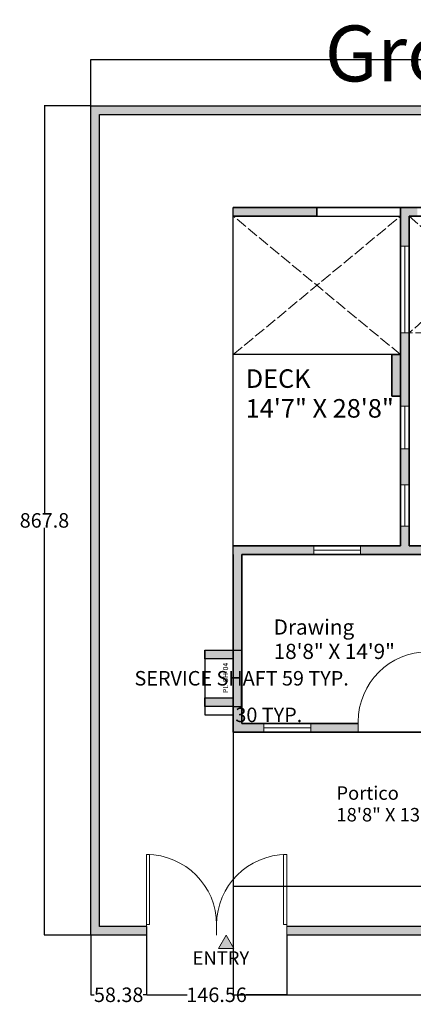
# Model space of a CAD drawing. Units: inches. Extents: x -828 to 1568, y -491 to 539.
# Tile 1 of 6: x -828 to -416, y -491 to 539. Entities that reach past the tile are written whole.
import ezdxf

# ---------------------------------------------------------------- set-up
doc = ezdxf.new("R2010")
doc.units = ezdxf.units.IN
doc.header["$MEASUREMENT"] = 0
doc.linetypes.add('ACAD_ISO02W100', pattern=[15, 12, -3])
for name, color, linetype, lineweight in [('A-ANNO-DIMS', 2, 'Continuous', 18), ('A-ANNO-SYMB', 7, 'Continuous', 18), ('A-ANNO-TEXT', 7, 'Continuous', 18), ('A-ANNO-TITL', 7, 'Continuous', 35), ('A-AREA-IDEN', 7, 'Continuous', 18), ('A-DOOR', 3, 'Continuous', 18), ('A-FLOR-EDGE', 7, 'Continuous', 25), ('A-FLOR-OVHD', 116, 'ACAD_ISO02W100', 13), ('A-FLOR-SHFT', 7, 'Continuous', 25), ('A-GLAZ', 4, 'Continuous', 18), ('A-WALL', 7, 'Continuous', 35), ('A-WALL-PATT', 8, 'Continuous', 13), ('L-SITE-GATE', 3, 'Continuous', 18), ('L-SITE-PATT', 8, 'Continuous', 13), ('L-SITE-WALL', 7, 'Continuous', 30)]:
    doc.layers.add(name, color=color, linetype=linetype, lineweight=lineweight)
doc.styles.get("Standard").update_dxf_attribs({"font": 'arial.ttf'})
doc.dimstyles.get("Standard").update_dxf_attribs({"dimtxt": 15.18, "dimasz": 0.18, "dimexe": 0.18, "dimexo": 0.0625, "dimgap": 0.09, "dimtad": 0, "dimtih": 1, "dimtoh": 1, "dimdec": 0, "dimzin": 0, "dimdsep": 46, "dimlunit": 3, "dimtxsty": 'Standard', "dimcen": 0.09, "dimadec": 0, "dimazin": 0, "dimtfac": 1, "dimtdec": 0, "dimtofl": 0, "dimtmove": 0, "dimatfit": 3, "dimfxl": 1, "dimtolj": 1, "dimtzin": 0, "dimarcsym": 0})

# ---------------------------------------------------------------- blocks, each defined once
blk = doc.blocks.new('*U2')
for p, q in [((0, 0), (0, -6)), ((40, 0), (40, -6))]:
    blk.add_line(p, q)
blk.add_lwpolyline([(0, 0), (0, 40), (1.75, 40), (1.75, 0)], close=True)
blk.add_arc((0, 0), 40, 0, 90)
blk = doc.blocks.new('SERVICE-SHAFT-59')
for p, q in [((0, 49.8), (0, 59)), ((0, 59), (29.6, 59)), ((0, 59), (0, 0)), ((29.6, 49.8), (0, 49.8)), ((0, 0), (0, 9)), ((0, 9), (29.6, 9)), ((29.6, 0), (0, 0))]:
    blk.add_line(p, q)
blk = doc.blocks.new('*D21')
at = {"layer": 'A-ANNO-DIMS', "color": 0, "lineweight": -2, "transparency": 16777216}
for p, q in [((-604.5, -120.5), (-595.5, -120.5)), ((-595.7, -120.6), (-595.7, -142)), ((-595.7, -179.3), (-595.7, -157.9)), ((-604.5, -179.4), (-595.5, -179.4))]:
    blk.add_line(p, q, dxfattribs=at)
at = {"layer": 'A-ANNO-DIMS', "color": 0, "lineweight": 20, "transparency": 16777216}
for points in [[(-595.7, -120.6), (-595.7, -120.6), (-595.7, -120.5)], [(-595.7, -179.3), (-595.7, -179.3), (-595.7, -179.4)]]:
    blk.add_solid(points, dxfattribs=at)
at = {"layer": 'DEFPOINTS', "color": 0, "lineweight": 20, "transparency": 16777216}
for p in [(-604.5, -120.5), (-595.7, -120.5), (-604.5, -179.4)]:
    blk.add_point(p, dxfattribs=at)
at = {"layer": 'A-ANNO-DIMS', "color": 0, "transparency": 16777216, "insert": (-595.7, -150), "char_height": 15.18, "attachment_point": 5}
blk.add_mtext('\\A1;SERVICE SHAFT 59 TYP.', dxfattribs=at)
blk = doc.blocks.new('*D22')
at = {"layer": 'A-ANNO-DIMS', "color": 0, "lineweight": -2, "transparency": 16777216}
for p, q in [((-634.1, -179.5), (-634.1, -188.5)), ((-604.5, -179.5), (-604.5, -188.5)), ((-633.9, -188.3), (-604.7, -188.3)), ((-604.5, -188.3), (-604.4, -188.3))]:
    blk.add_line(p, q, dxfattribs=at)
at = {"layer": 'A-ANNO-DIMS', "color": 0, "lineweight": 20, "transparency": 16777216}
for points in [[(-633.9, -188.3), (-633.9, -188.3), (-634.1, -188.3)], [(-604.7, -188.3), (-604.7, -188.3), (-604.5, -188.3)]]:
    blk.add_solid(points, dxfattribs=at)
at = {"layer": 'DEFPOINTS', "color": 0, "lineweight": 20, "transparency": 16777216}
for p in [(-634.1, -179.4), (-604.5, -179.4), (-604.5, -188.3)]:
    blk.add_point(p, dxfattribs=at)
at = {"layer": 'A-ANNO-DIMS', "color": 0, "transparency": 16777216, "insert": (-567.3, -188.3), "char_height": 15.18, "attachment_point": 5}
blk.add_mtext('\\A1;30 TYP.', dxfattribs=at)
blk = doc.blocks.new('*D31')
at = {"layer": 'A-ANNO-DIMS', "color": 0, "lineweight": -2, "transparency": 16777216}
for p, q in [((-753.5, 449.1), (-753.5, 497.6)), ((-753.3, 497.4), (-321.9, 497.4)), ((143.3, 497.4), (-288.2, 497.4)), ((143.5, 449.1), (143.5, 497.6))]:
    blk.add_line(p, q, dxfattribs=at)
at = {"layer": 'A-ANNO-DIMS', "color": 0, "lineweight": 20, "transparency": 16777216}
for points in [[(-753.3, 497.5), (-753.3, 497.4), (-753.5, 497.4)], [(143.3, 497.5), (143.3, 497.4), (143.5, 497.4)]]:
    blk.add_solid(points, dxfattribs=at)
at = {"layer": 'DEFPOINTS', "color": 0, "lineweight": 20, "transparency": 16777216}
for p in [(143.5, 497.4), (-753.5, 449), (143.5, 449)]:
    blk.add_point(p, dxfattribs=at)
at = {"layer": 'A-ANNO-DIMS', "color": 0, "transparency": 16777216, "insert": (-305, 497.4), "char_height": 15.18, "attachment_point": 5}
blk.add_mtext('\\A1;897', dxfattribs=at)
blk = doc.blocks.new('*D32')
at = {"layer": 'A-ANNO-DIMS', "color": 0, "lineweight": -2, "transparency": 16777216}
for p, q in [((-753.6, 449), (-802.1, 449)), ((-801.9, 448.9), (-801.9, 23)), ((-801.9, -418.6), (-801.9, 7.3)), ((-753.6, -418.7), (-802.1, -418.7))]:
    blk.add_line(p, q, dxfattribs=at)
at = {"layer": 'A-ANNO-DIMS', "color": 0, "lineweight": 20, "transparency": 16777216}
for points in [[(-801.9, 448.9), (-801.9, 448.9), (-801.9, 449)], [(-801.9, -418.6), (-801.9, -418.6), (-801.9, -418.7)]]:
    blk.add_solid(points, dxfattribs=at)
at = {"layer": 'DEFPOINTS', "color": 0, "lineweight": 20, "transparency": 16777216}
for p in [(-801.9, 449), (-753.5, 449), (-753.5, -418.7)]:
    blk.add_point(p, dxfattribs=at)
at = {"layer": 'A-ANNO-DIMS', "color": 0, "transparency": 16777216, "insert": (-801.9, 15.2), "char_height": 15.18, "attachment_point": 5}
blk.add_mtext('\\A1;867.8', dxfattribs=at)
blk = doc.blocks.new('*D33')
at = {"layer": 'A-ANNO-DIMS', "color": 0, "lineweight": -2, "transparency": 16777216}
for p, q in [((-604.5, -367.5), (-604.5, -481.4)), ((26.5, -367.5), (26.5, -481.4)), ((-604.4, -481.2), (-304.5, -481.2)), ((26.3, -481.2), (-273.6, -481.2))]:
    blk.add_line(p, q, dxfattribs=at)
at = {"layer": 'A-ANNO-DIMS', "color": 0, "lineweight": 20, "transparency": 16777216}
for points in [[(-604.4, -481.2), (-604.4, -481.2), (-604.5, -481.2)], [(26.3, -481.2), (26.3, -481.2), (26.5, -481.2)]]:
    blk.add_solid(points, dxfattribs=at)
at = {"layer": 'DEFPOINTS', "color": 0, "lineweight": 20, "transparency": 16777216}
for p in [(-604.5, -367.4), (26.5, -367.4), (26.5, -481.2)]:
    blk.add_point(p, dxfattribs=at)
at = {"layer": 'A-ANNO-DIMS', "color": 0, "transparency": 16777216, "insert": (-289, -481.2), "char_height": 15.18, "attachment_point": 5}
blk.add_mtext('\\A1;631', dxfattribs=at)
blk = doc.blocks.new('*D37')
at = {"layer": 'A-ANNO-DIMS', "color": 0, "lineweight": -2, "transparency": 16777216}
for p, q in [((-695.1, -418.8), (-695.1, -481.4)), ((-548.6, -418.8), (-548.6, -481.4)), ((-695, -481.2), (-652.7, -481.2)), ((-548.8, -481.2), (-591, -481.2))]:
    blk.add_line(p, q, dxfattribs=at)
at = {"layer": 'A-ANNO-DIMS', "color": 0, "lineweight": 20, "transparency": 16777216}
for points in [[(-695, -481.2), (-695, -481.2), (-695.1, -481.2)], [(-548.8, -481.2), (-548.8, -481.2), (-548.6, -481.2)]]:
    blk.add_solid(points, dxfattribs=at)
at = {"layer": 'DEFPOINTS', "color": 0, "lineweight": 20, "transparency": 16777216}
for p in [(-695.1, -418.7), (-548.6, -418.7), (-548.6, -481.2)]:
    blk.add_point(p, dxfattribs=at)
at = {"layer": 'A-ANNO-DIMS', "color": 0, "transparency": 16777216, "insert": (-621.9, -481.2), "char_height": 15.18, "attachment_point": 5}
blk.add_mtext('\\A1;146.56', dxfattribs=at)
blk = doc.blocks.new('*D38')
at = {"layer": 'A-ANNO-DIMS', "color": 0, "lineweight": -2, "transparency": 16777216}
for p, q in [((-753.5, -418.8), (-753.5, -481.4)), ((-695.1, -418.8), (-695.1, -481.4)), ((-753.3, -481.2), (-750, -481.2)), ((-695.3, -481.2), (-698.6, -481.2))]:
    blk.add_line(p, q, dxfattribs=at)
at = {"layer": 'A-ANNO-DIMS', "color": 0, "lineweight": 20, "transparency": 16777216}
for points in [[(-753.3, -481.2), (-753.3, -481.2), (-753.5, -481.2)], [(-695.3, -481.2), (-695.3, -481.2), (-695.1, -481.2)]]:
    blk.add_solid(points, dxfattribs=at)
at = {"layer": 'DEFPOINTS', "color": 0, "lineweight": 20, "transparency": 16777216}
for p in [(-753.5, -418.7), (-695.1, -418.7), (-695.1, -481.2)]:
    blk.add_point(p, dxfattribs=at)
at = {"layer": 'A-ANNO-DIMS', "color": 0, "transparency": 16777216, "insert": (-724.3, -481.2), "char_height": 15.18, "attachment_point": 5}
blk.add_mtext('\\A1;58.38', dxfattribs=at)

msp = doc.modelspace()

# ---------------------------------------------------------------- hatches: boundary and pattern name
at = {"layer": 'A-ANNO-SYMB'}
h = msp.add_hatch(color=256, dxfattribs=at)
h.dxf.hatch_style = 1
h.paths.add_polyline_path([(-611.9024, -418.9253), (-619.9125, -432.7993), (-603.8922, -432.7993)])
at = {"layer": 'A-WALL-PATT'}
h = msp.add_hatch(color=256, dxfattribs=at)
h.dxf.hatch_style = 1
h.paths.add_polyline_path([(-473.7903, -197.4155), (-523.4337, -197.4155), (-523.4337, -206.4155), (-473.7903, -206.4155)])
h.paths.add_polyline_path([(-572.3651, -197.4155), (-595.5391, -197.4155), (-595.5391, -20.4155), (-520.2134, -20.4155), (-520.2134, -11.4155), (-604.5391, -11.4155), (-604.5391, -206.4155), (-572.3651, -206.4155)])
h.paths.add_polyline_path([(-604.5391, -170.4394), (-634.1027, -170.4394), (-634.1027, -179.4394), (-604.5391, -179.4394)])
h.paths.add_polyline_path([(-604.5391, -120.4631), (-634.1027, -120.4631), (-634.1027, -129.6673), (-604.5391, -129.6673)])
h.paths.add_polyline_path([(-268.3198, -11.4155), (-420.5391, -11.4155), (-420.5391, 9.0334), (-429.5391, 9.0334), (-429.5391, -11.4155), (-471.2821, -11.4155), (-471.2821, -20.4155), (-371.5391, -20.4155), (-371.5391, -197.4155), (-400.5108, -197.4155), (-400.5108, -206.4155), (-371.5391, -206.4155), (-371.5391, -282.4155), (-367.0391, -282.4155), (-362.5391, -282.4155), (-362.5391, -122.4155), (-313.1564, -122.4155), (-313.1564, -113.4155), (-362.5391, -113.4155), (-362.5391, -20.4155), (-268.3198, -20.4155)])
h.paths.add_polyline_path([(-313.539, 165.5845), (-375.5295, 165.5845), (-375.5295, 159.5845), (-313.539, 159.5845)])
h.paths.add_polyline_path([(-420.5391, 90.211), (-429.5391, 90.211), (-429.5391, 52.4437), (-420.5391, 52.4437)])
h.paths.add_polyline_path([(-420.5391, 211.3197), (-429.5391, 211.3197), (-429.5391, 134.8496), (-425.0391, 134.8496), (-420.5391, 134.8496), (-420.5391, 165.5845)])
h.paths.add_polyline_path([(-429.5391, 188.7113), (-438.5391, 188.7113), (-438.5391, 145.3797), (-429.5391, 145.3797)])
h.paths.add_polyline_path([(-517.0391, 342.5845), (-604.5391, 342.5845), (-604.5391, 333.5845), (-517.0391, 333.5845)])
h.paths.add_polyline_path([(-411.8784, 342.5845), (-429.5391, 342.5845), (-429.5391, 302.1645), (-420.5391, 302.1645), (-420.5391, 333.5845), (-411.8784, 333.5845)])
h.paths.add_polyline_path([(-311.8294, 372.1481), (-321.0336, 372.1481), (-321.0336, 342.5845), (-311.8294, 342.5845)])
h.paths.add_polyline_path([(-282.0163, 372.1481), (-291.2206, 372.1481), (-291.2206, 342.5845), (-282.0163, 342.5845)])
h.paths.add_polyline_path([(-230.7265, 342.5845), (-321.0336, 342.5845), (-321.0336, 333.5845), (-230.7265, 333.5845)])
h.paths.add_polyline_path([(-23.3113, 372.1481), (-32.5155, 372.1481), (-32.5155, 342.5845), (-23.3113, 342.5845)])
h.paths.add_polyline_path([(26.4609, 372.1481), (17.4609, 372.1481), (17.4609, 342.5845), (26.4609, 342.5845)])
h.paths.add_polyline_path([(56.6461, 259.1031), (26.4609, 259.1031), (26.4609, 248.5663), (56.6461, 248.5663)])
h.paths.add_polyline_path([(56.6461, 216.517), (26.4609, 216.517), (26.4609, 206.4193), (56.6461, 206.4193)])
h.paths.add_polyline_path([(56.0244, -54.4391), (26.4609, -54.4391), (26.4609, -63.6433), (56.0244, -63.6433)])
h.paths.add_polyline_path([(56.0244, -163.1876), (26.4609, -163.1876), (26.4609, -172.3918), (56.0244, -172.3918)])
h.paths.add_polyline_path([(56.0244, -113.4155), (56.0244, -104.4155), (26.4609, -104.4155), (26.4609, -122.4155), (56.0244, -122.4155)])
h.paths.add_polyline_path([(-23.844, -367.4155), (-134.8372, -367.4155), (-134.8372, -376.4155), (-23.844, -376.4155)])
h.paths.add_polyline_path([(26.4609, -54.4391), (21.9609, -54.4391), (17.4609, -54.4391), (17.4609, -113.4155), (-252.861, -113.4155), (-252.861, -122.4155), (-69.5391, -122.4155), (-69.5391, -282.9566), (-65.5391, -282.9566), (-65.5391, -250.4155), (-53.4738, -250.4155), (-53.4738, -246.4155), (-65.5391, -246.4155), (-65.5391, -122.4155), (17.4609, -122.4155), (17.4609, -172.3918), (26.4609, -172.3918), (26.4609, -163.1876)])
h.paths.add_polyline_path([(-172.5391, 156.5845), (-97.5391, 156.5845), (-97.5391, 62.5845), (-172.5391, 62.5845), (-172.5391, 98.9611, -0.058998616), (-178.0193, 98.3122), (-181.5391, 98.3122), (-181.5391, 33.9683), (-172.5391, 33.9683), (-172.5391, 53.5845), (-97.5391, 53.5845), (-97.5391, -11.4155), (-172.5391, -11.4155), (-172.5391, 9.9791), (-181.5391, 9.9791), (-181.5391, -11.4155), (-181.5391, -20.4155), (17.4609, -20.4155), (17.4609, -29.0707), (26.4609, -29.0707), (26.4609, 17.0407), (17.4609, 17.0407), (17.4609, -11.4155), (-88.5391, -11.4155), (-88.5391, 82.5845), (17.4609, 82.5845), (17.4609, 68.3133), (22.9411, 68.3133), (26.4609, 68.3133), (26.4609, 113.8123), (23.0131, 113.8123), (17.4609, 113.8123), (17.4609, 91.5845), (-88.5391, 91.5845), (-88.5391, 156.5845), (17.4609, 156.5845), (17.4609, 136.6113, -0.059791184), (23.0131, 137.2776), (26.4609, 137.2776), (26.4609, 259.1031), (21.9609, 259.1031), (17.4609, 259.1031), (17.4609, 237.5845), (-88.5391, 237.5845), (-88.5391, 249.5845), (-94.0193, 249.5845), (-97.5391, 249.5845), (-97.5391, 217.6678), (-94.0193, 217.6678), (-88.5391, 217.6678), (-88.5391, 230.5845), (17.4609, 230.5845), (17.4609, 165.5845), (-88.5391, 165.5845), (-88.5391, 194.8514, -0.058998616), (-94.0193, 194.2024), (-97.5391, 194.2024), (-97.5391, 165.5845), (-276.9691, 165.5845), (-276.9691, 156.5845), (-181.5391, 156.5845), (-181.5391, 121.7776), (-178.0193, 121.7776), (-172.5391, 121.7776)])
h.paths.add_polyline_path([(-88.5391, 333.5845), (17.4609, 333.5845), (17.4609, 313.1897), (26.4609, 313.1897), (26.4609, 342.5845), (-139.8817, 342.5845), (-139.8817, 333.5845), (-97.5391, 333.5845), (-97.5391, 273.0499), (-94.0193, 273.0499, -0.058998616), (-88.5391, 272.401)])
h.paths.add_polyline_path([(26.4609, -232.3042), (17.4609, -232.3042), (17.4609, -246.4155), (-35.2489, -246.4155), (-35.2489, -250.4155), (17.4609, -250.4155), (17.4609, -358.4155), (-65.5391, -358.4155), (-65.5391, -311.3725), (-69.5391, -311.3725), (-69.5391, -358.4155), (-261.1271, -358.4155), (-261.1271, -367.4155), (26.4609, -367.4155)])
at = {"layer": 'L-SITE-PATT'}
h = msp.add_hatch(color=256, dxfattribs=at)
h.dxf.hatch_style = 1
h.paths.add_polyline_path([(-695.1383, -418.734), (-695.1383, -409.734), (-744.5156, -409.734), (-744.5156, 440.0429), (134.4735, 440.0429), (134.4735, -409.734), (-428.0987, -409.734), (-428.0987, -418.734), (143.4735, -418.734), (143.4735, 449.0429), (-753.5156, 449.0429), (-753.5156, -418.734)])
h = msp.add_hatch(color=256, dxfattribs=at)
h.dxf.hatch_style = 1
h.paths.add_polyline_path([(-428.0987, -409.734), (-548.5793, -409.734), (-548.5793, -418.734), (-428.0987, -418.734)])

# ---------------------------------------------------------------- linework, layer by layer
at = {"layer": 'A-ANNO-SYMB'}
msp.add_lwpolyline([(-611.9024, -418.9253), (-619.9125, -432.7993), (-603.8922, -432.7993)], close=True, dxfattribs=at)
at = {"layer": 'A-FLOR-EDGE'}
for p, q in [((-604.5391, -11.4155), (-604.5391, 342.5845)), ((-604.5391, 333.5845), (-429.5391, 333.5845)), ((-517.0391, 333.5845), (-429.5391, 333.5845)), ((-429.5391, 333.5845), (-429.5391, 188.7113)), ((-429.5391, 333.5845), (-429.5391, 188.7113)), ((-429.5391, 188.7113), (-604.5391, 188.7113)), ((-604.5391, -20.4155), (-604.5391, -11.4155)), ((-604.5391, -206.4155), (-604.5391, -367.4155)), ((-604.5391, -367.4155), (-371.5391, -367.4155))]:
    msp.add_line(p, q, dxfattribs=at)
at = {"layer": 'A-FLOR-OVHD'}
for p, q in [((-604.5391, 188.7113), (-429.5391, 333.5845)), ((-429.5391, 188.7113), (-604.5391, 333.5845)), ((-420.5391, 211.3197), (-420.5391, 333.5845)), ((-420.5391, 333.5845), (-282.0163, 333.5845)), ((-282.0163, 333.5845), (-420.5391, 211.3197)), ((-420.5391, 211.3197), (-420.5391, 333.5845)), ((-420.5391, 333.5845), (-282.0163, 211.3197)), ((-282.0163, 211.3197), (-420.5391, 211.3197))]:
    msp.add_line(p, q, dxfattribs=at)
at = {"layer": 'A-GLAZ'}
for p, q in [((-420.5391, 302.1645), (-429.5391, 302.1645)), ((-429.5391, 302.1645), (-429.5391, 211.3197)), ((-425.0391, 211.3197), (-425.0391, 302.1645)), ((-420.5391, 211.3197), (-420.5391, 302.1645)), ((-429.5391, 211.3197), (-420.5391, 211.3197)), ((-429.5391, 211.3197), (-425.0391, 211.3197)), ((-429.5391, 134.8496), (-420.5391, 134.8496)), ((-429.5391, 90.211), (-429.5391, 134.8496)), ((-429.5391, 134.8496), (-425.0391, 134.8496)), ((-425.0391, 134.8496), (-425.0391, 90.211)), ((-420.5391, 134.8496), (-420.5391, 90.211)), ((-420.5391, 90.211), (-429.5391, 90.211)), ((-420.5391, 52.4437), (-429.5391, 52.4437)), ((-429.5391, 52.4437), (-429.5391, 9.0334)), ((-425.0391, 9.0334), (-425.0391, 52.4437)), ((-420.5391, 9.0334), (-420.5391, 52.4437)), ((-429.5391, 9.0334), (-420.5391, 9.0334)), ((-429.5391, 9.0334), (-425.0391, 9.0334)), ((-471.2821, -11.4155), (-520.2134, -11.4155)), ((-520.2134, -11.4155), (-520.2134, -20.4155)), ((-471.2821, -15.9155), (-520.2134, -15.9155)), ((-520.2134, -20.4155), (-471.2821, -20.4155)), ((-471.2821, -20.4155), (-471.2821, -11.4155)), ((-523.4337, -197.4155), (-572.3651, -197.4155)), ((-572.3651, -197.4155), (-572.3651, -206.4155)), ((-523.4337, -201.9155), (-572.3651, -201.9155)), ((-523.4337, -206.4155), (-523.4337, -197.4155)), ((-523.4337, -206.4155), (-523.4337, -201.9155)), ((-572.3651, -206.4155), (-523.4337, -206.4155))]:
    msp.add_line(p, q, dxfattribs=at)
at = {"layer": 'A-WALL'}
for p, q in [((-517.0391, 342.5845), (-604.5391, 342.5845)), ((-517.0391, 333.5845), (-517.0391, 342.5845)), ((-429.5391, 342.5845), (-517.0391, 342.5845)), ((26.4609, 342.5845), (-429.5391, 342.5845)), ((-429.5391, 342.5845), (-429.5391, -11.4155)), ((-517.0391, 333.5845), (-604.5391, 333.5845)), ((-429.5391, 333.5845), (-429.5391, 165.5845)), ((-420.5391, 333.5845), (-420.5391, 165.5845)), ((-97.5391, 333.5845), (-420.5391, 333.5845)), ((-429.5391, 188.7113), (-438.5391, 188.7113)), ((-438.5391, 188.7113), (-438.5391, 145.3797)), ((-429.5391, 192.7156), (-429.5391, 165.5845)), ((-420.5391, 165.5845), (-420.5391, -11.4155)), ((-438.5391, 145.3797), (-429.5391, 145.3797)), ((-604.5391, -11.4155), (-429.5391, -11.4155)), ((-604.5391, -20.4155), (-604.5391, -206.4155)), ((-595.5391, -20.4155), (-429.5391, -20.4155)), ((-595.5391, -20.4155), (-371.5391, -20.4155)), ((-595.5391, -20.4155), (-595.5391, -197.4155)), ((-595.5391, -20.4155), (-371.5391, -20.4155)), ((-420.5391, -11.4155), (-268.3198, -11.4155)), ((-595.5391, -197.4155), (-473.7903, -197.4155)), ((-604.5391, -206.4155), (-371.5391, -206.4155))]:
    msp.add_line(p, q, dxfattribs=at)
at = {"layer": 'L-SITE-WALL'}
msp.add_line((-695.1383, -409.734), (-695.1383, -418.734), dxfattribs=at)
for points in [[(-695.1383, -418.734), (-753.5156, -418.734), (-753.5156, 449.0429), (143.4735, 449.0429), (143.4735, -418.734), (-548.5793, -418.734)], [(-695.1383, -409.734), (-744.5156, -409.734), (-744.5156, 440.0429), (134.4735, 440.0429), (134.4735, -409.734), (-548.5793, -409.734)]]:
    msp.add_lwpolyline(points, dxfattribs=at)

# ---------------------------------------------------------------- block references
at = {"layer": 'A-DOOR', "xscale": -1.831987710751254, "yscale": 1.831987710751254, "zscale": 1.831987710751254}
msp.add_blockref('*U2', (-400.5108, -195.4235), dxfattribs=at)
at = {"layer": 'A-FLOR-SHFT'}
msp.add_blockref('SERVICE-SHAFT-59', (-634.103, -179.439), dxfattribs=at)
at = {"layer": 'L-SITE-GATE', "yscale": 1.831987710751254, "zscale": 1.831987710751254}
for p, xscale in [((-695.1383, -407.7421), 1.831987710751254), ((-548.5793, -407.7421), -1.831987710751254)]:
    msp.add_blockref('*U2', p, dxfattribs=dict(at, xscale=xscale))

# ---------------------------------------------------------------- texts
at = {"layer": 'A-ANNO-TEXT'}
msp.add_text('PL-SH-04', height=5.4126, rotation=90, dxfattribs=at).set_placement((-609.8571, -165.4609))
msp.add_text('ENTRY', height=14.09928, dxfattribs=at).set_placement((-646.9761, -449.8192))
at = {"layer": 'A-ANNO-TITL'}
msp.add_text('Ground floor', height=58.547339, dxfattribs=at).set_placement((-508.7568, 474.5437))
at = {"layer": 'A-AREA-IDEN'}
for s, height, p in [('DECK', 19.3914, (-591.4227, 153.8995)), ('14\'7" X 28\'8"', 19.3914, (-591.4227, 122.7489)), ('Drawing', 15.8724, (-562.201, -104.3054)), ('18\'8" X 14\'9"', 15.872402, (-562.201, -129.803)), ('Portico', 14.09928, (-496.6166, -277.1704)), ('18\'8" X 13\'0"', 14.099277, (-496.6166, -299.8197))]:
    msp.add_text(s, height=height, dxfattribs=at).set_placement(p)

# ---------------------------------------------------------------- dimensions: what is measured, and where the dimension line sits
at = {"layer": 'A-ANNO-DIMS'}
for base, p1, p2, override, picture, middle in [((143.4735, 497.4429), (-753.5156, 449.0429), (143.4735, 449.0429), {"dimdec": 0, "dimlfac": 1, "dimrnd": 0, "dimzin": 0, "dimdsep": 46, "dimlunit": 2}, '*D31', (-305.0211, 497.4429)), ((26.4609, -481.1993), (-604.5391, -367.4155), (26.4609, -367.4155), {"dimdec": 0, "dimlfac": 1, "dimrnd": 0, "dimzin": 0, "dimdsep": 46, "dimlunit": 2}, '*D33', (-289.0391, -481.1993)), ((-695.1383, -481.1993), (-753.5156, -418.734), (-695.1383, -418.734), {"dimdec": 2, "dimlfac": 1, "dimrnd": 0, "dimzin": 0, "dimdsep": 46, "dimlunit": 2}, '*D38', (-724.3269, -481.1993)), ((-548.5793, -481.1993), (-695.1383, -418.734), (-548.5793, -418.734), {"dimdec": 2, "dimlfac": 1, "dimrnd": 0, "dimzin": 0, "dimdsep": 46, "dimlunit": 2}, '*D37', (-621.8588, -481.1993))]:
    dim = msp.add_linear_dim(base=base, p1=p1, p2=p2, dimstyle='Standard', override=override, dxfattribs=at)
    dim.commit()
    dim.dimension.update_dxf_attribs({"geometry": picture, "text_midpoint": middle})
dim = msp.add_linear_dim(base=(-801.9156, 449.0429), p1=(-753.5156, -418.734), p2=(-753.5156, 449.0429), angle=90, dimstyle='Standard', override={"dimdec": 1, "dimlfac": 1, "dimrnd": 0, "dimzin": 0, "dimdsep": 46, "dimlunit": 2}, dxfattribs=at)
dim.commit()
dim.dimension.update_dxf_attribs({"geometry": '*D32', "text_midpoint": (-801.9156, 15.1544)})
dim = msp.add_linear_dim(base=(-595.6927, -120.4631), p1=(-604.5391, -179.4394), p2=(-604.5391, -120.4631), angle=90, text='SERVICE SHAFT <> TYP.', dimstyle='Standard', override={"dimdec": 0, "dimlfac": 1, "dimrnd": 0, "dimzin": 0, "dimdsep": 46, "dimlunit": 2}, dxfattribs=at)
dim.commit()
dim.dimension.update_dxf_attribs({"geometry": '*D21', "text_midpoint": (-595.6927, -149.9512)})
dim = msp.add_linear_dim(base=(-604.5391, -188.2859), p1=(-634.1027, -179.4394), p2=(-604.5391, -179.4394), text='<> TYP.', dimstyle='Standard', override={"dimdec": 0, "dimlfac": 1, "dimrnd": 0, "dimzin": 0, "dimdsep": 46, "dimlunit": 2}, dxfattribs=at)
dim.commit()
dim.dimension.update_dxf_attribs({"geometry": '*D22', "text_midpoint": (-567.3287, -188.2859)})

doc.saveas('drawing.dxf')
